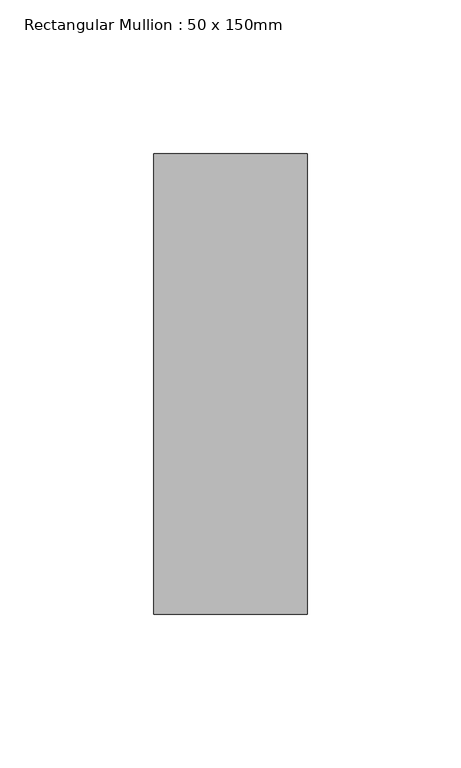
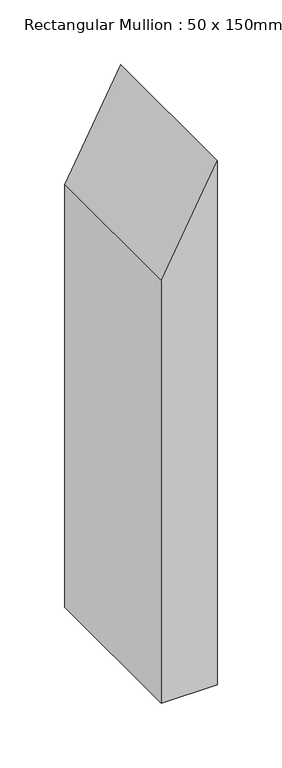
"""IFC4 building model written with IfcOpenShell, lengths in millimetres: member geometry, Rectangular Mullion : 50 x 150mm."""

from ifc_helpers import new_model, si_unit, frame, origin, place, context, project, spatial, polyline, outline, extrude, source, transform, mapped, element, save


def rectangular_mullion_50_x_150mm_17c629a1(model_context):
    return source(origin(), model_context, "Body", "SweptSolid", [
        extrude(outline(polyline([(0.0, 0.0), (-96.0491063, -50.0), (-495.3320611, -50.0), (-495.3320611, 0.0), (0.0, 0.0)])), frame((0.0, -75.0, 0.0), z_axis=(0.0, 1.0, 0.0), x_axis=(0.0, 0.0, 1.0)), (0.0, 0.0, 1.0), 150.0),
    ])


if __name__ == "__main__":
    model = new_model("IFC4")
    model_context = context("Model", 3, world=origin())
    ifc_project = project(units=[si_unit("LENGTHUNIT", "METRE", prefix="MILLI")], contexts=[model_context])
    site = spatial("IfcSite", under=ifc_project)
    building = spatial("IfcBuilding", under=site)
    placement = place(None, origin())
    rectangular_mullion_50_x_150mm_shape = rectangular_mullion_50_x_150mm_17c629a1(model_context)
    element("IfcMember", 1, ObjectType="Rectangular Mullion : 50 x 150mm", at=placement, inside=building, context=model_context, shape_type="MappedRepresentation", body=[
        mapped(rectangular_mullion_50_x_150mm_shape, transform((0.0, 0.0, 0.0), x_axis=(1.0, 0.0, 0.0), y_axis=(0.0, 1.0, 0.0), z_axis=(0.0, 0.0, 1.0))),
    ])
    save(model, "model.ifc")

# Revit data of these elements
# Type "Rectangular Mullion : 50 x 150mm"
#   built-in parameter 1007304 = 0.492126 (stored number, unit not read)
#   built-in parameter 1007301 = 0.082021 (stored number, unit not read)
#   built-in parameter 1007300 = 0.082021 (stored number, unit not read)
# Element 1 (IfcMember, "Rectangular Mullion : 50 x 150mm")
#   Materials on its faces: "Aluminium"
# Materials
#   "Aluminium": class "Metal", colour RGB 247 247 247, transparency 0, Description = "Aluminium 6061", Cost = 0
